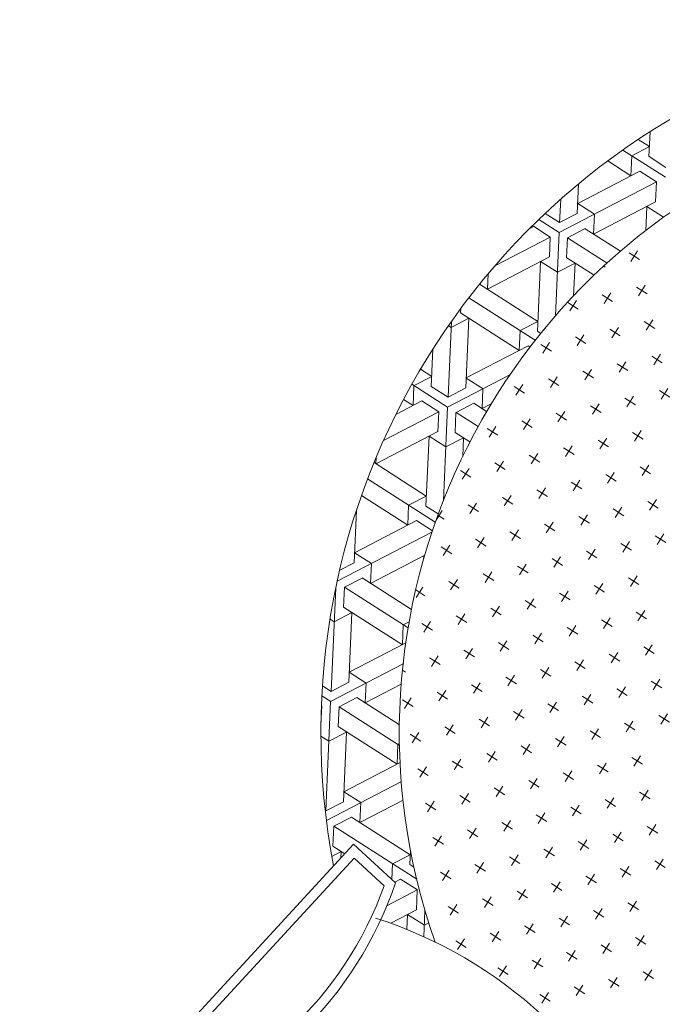
# Model space of a CAD drawing. Units: inches. Extents: x -4843 to -3402, y -164 to 3629.
# Tile 11 of 22: x -4530 to -4506, y 864 to 900. Entities that reach past the tile are written whole.
import ezdxf

# ---------------------------------------------------------------- set-up
doc = ezdxf.new("R2010")
doc.units = ezdxf.units.IN
doc.layers.add('furniture', color=6, linetype='Continuous', lineweight=18)

# ---------------------------------------------------------------- blocks, each defined once
blk = doc.blocks.new('A$C30AE1D3B')
for p, q in [((2071.5, 1090.4, -685.7), (2054.2, 1082.4, -685.7)), ((2066.8, 1077.8, -685.7), (2058.8, 1095.1, -685.7)), ((2122.1, 1072, -685.7), (2104.8, 1064, -685.7)), ((2117.5, 1059.4, -685.7), (2109.4, 1076.6, -685.7)), ((2172.7, 1053.6, -685.7), (2155.5, 1045.5, -685.7)), ((2168.1, 1040.9, -685.7), (2160.1, 1058.2, -685.7)), ((2053, 1039.8, -685.7), (2035.8, 1031.8, -685.7)), ((2048.4, 1027.2, -685.7), (2040.4, 1044.4, -685.7)), ((2218.7, 1022.5, -685.7), (2210.7, 1039.8, -685.7)), ((2099.1, 1008.7, -685.7), (2091, 1026, -685.7)), ((2223.4, 1035.2, -685.7), (2206.1, 1027.1, -685.7)), ((2103.7, 1021.4, -685.7), (2086.4, 1013.3, -685.7)), ((2030, 976.5, -685.7), (2021.9, 993.8, -685.7)), ((2154.3, 1003, -685.7), (2137, 994.9, -685.7)), ((2149.7, 990.3, -685.7), (2141.6, 1007.6, -685.7)), ((2034.6, 989.2, -685.7), (2017.3, 981.1, -685.7)), ((2204.9, 984.5, -685.7), (2187.7, 976.5, -685.7)), ((2200.3, 971.9, -685.7), (2192.3, 989.1, -685.7)), ((2085.2, 970.8, -685.7), (2068, 962.7, -685.7)), ((2080.6, 958.1, -685.7), (2072.6, 975.4, -685.7)), ((2255.6, 966.1, -685.7), (2238.3, 958, -685.7)), ((2250.9, 953.4, -685.7), (2242.9, 970.7, -685.7)), ((1965.5, 957, -685.7), (1948.3, 948.9, -685.7)), ((1960.9, 944.3, -685.7), (1952.9, 961.6, -685.7)), ((2135.9, 952.3, -685.7), (2118.6, 944.3, -685.7)), ((2131.3, 939.7, -685.7), (2123.2, 956.9, -685.7)), ((2016.2, 938.6, -685.7), (1998.9, 930.5, -685.7)), ((2011.6, 925.9, -685.7), (2003.5, 943.2, -685.7)), ((2186.5, 933.9, -685.7), (2169.2, 925.8, -685.7)), ((2181.9, 921.2, -685.7), (2173.8, 938.5, -685.7)), ((2066.8, 920.1, -685.7), (2049.5, 912.1, -685.7)), ((2062.2, 907.5, -685.7), (2054.1, 924.7, -685.7)), ((2232.5, 902.8, -685.7), (2224.5, 920.1, -685.7)), ((1947.1, 906.3, -685.7), (1929.8, 898.3, -685.7)), ((1942.5, 893.7, -685.7), (1934.4, 911, -685.7)), ((2112.8, 889, -685.7), (2104.8, 906.3, -685.7)), ((2237.1, 915.5, -685.7), (2219.9, 907.4, -685.7)), ((1997.7, 887.9, -685.7), (1980.5, 879.9, -685.7)), ((1993.1, 875.3, -685.7), (1985.1, 892.5, -685.7)), ((2117.4, 901.7, -685.7), (2100.2, 893.6, -685.7)), ((2163.5, 870.6, -685.7), (2155.4, 887.9, -685.7)), ((2287.8, 897, -685.7), (2270.5, 889, -685.7)), ((2283.2, 884.4, -685.7), (2275.1, 901.6, -685.7)), ((2043.8, 856.8, -685.7), (2035.7, 874.1, -685.7)), ((2168.1, 883.3, -685.7), (2150.8, 875.2, -685.7)), ((3045.6, 881, -685.7), (2346.6, 694.2, -685.7)), ((1924.1, 843.1, -685.7), (1916, 860.3, -685.7)), ((2048.4, 869.5, -685.7), (2031.1, 861.4, -685.7)), ((2218.7, 864.8, -685.7), (2201.4, 856.8, -685.7)), ((2214.1, 852.2, -685.7), (2206, 869.4, -685.7)), ((3064, 870.4, -685.7), (2336, 675.8, -685.7)), ((1928.7, 855.7, -685.7), (1911.4, 847.7, -685.7)), ((2099, 851.1, -685.7), (2081.7, 843, -685.7)), ((2094.4, 838.4, -685.7), (2086.3, 855.7, -685.7)), ((2269.3, 846.4, -685.7), (2252.1, 838.4, -685.7)), ((2264.7, 833.7, -685.7), (2256.7, 851, -685.7)), ((2298.2, 820.3, -685.7), (2321, 852.9, -685.7)), ((1979.3, 837.3, -685.7), (1962, 829.2, -685.7)), ((1974.7, 824.6, -685.7), (1966.7, 841.9, -685.7)), ((2149.6, 832.6, -685.7), (2132.4, 824.6, -685.7)), ((2145, 820, -685.7), (2137, 837.2, -685.7)), ((2310.8, 838.4, -685.7), (2303.4, 839.1, -685.7)), ((2310.8, 838.4, -685.7), (2323.7, 810.8, -685.7)), ((2336.8, 829.5, -685.7), (2323.7, 810.8, -685.7)), ((2029.9, 818.9, -685.7), (2012.7, 810.8, -685.7)), ((2025.3, 806.2, -685.7), (2017.3, 823.5, -685.7)), ((2200.3, 814.2, -685.7), (2183, 806.2, -685.7)), ((2195.7, 801.5, -685.7), (2187.6, 818.8, -685.7)), ((1910.3, 805.1, -685.7), (1893, 797, -685.7)), ((1905.6, 792.4, -685.7), (1897.6, 809.7, -685.7)), ((2080.6, 800.4, -685.7), (2063.3, 792.4, -685.7)), ((2076, 787.8, -685.7), (2067.9, 805, -685.7)), ((2246.3, 783.1, -685.7), (2238.2, 800.4, -685.7)), ((2291.1, 787.2, -685.7), (2308.5, 812.1, -685.7)), ((2308.5, 812.1, -685.7), (2352.6, 808.3, -685.7)), ((1960.9, 786.7, -685.7), (1943.6, 778.6, -685.7)), ((1956.3, 774, -685.7), (1948.2, 791.3, -685.7)), ((2126.6, 769.3, -685.7), (2118.5, 786.6, -685.7)), ((2250.9, 795.8, -685.7), (2233.6, 787.7, -685.7)), ((2291, 787.2, -685.7), (2303.9, 759.5, -685.7)), ((2343.1, 782.6, -685.7), (2291, 787.1, -685.7)), ((1841.2, 772.9, -685.7), (1823.9, 764.8, -685.7)), ((1836.6, 760.2, -685.7), (1828.5, 777.5, -685.7)), ((2011.5, 768.2, -685.7), (1994.2, 760.2, -685.7)), ((2006.9, 755.6, -685.7), (1998.9, 772.8, -685.7)), ((2131.2, 782, -685.7), (2113.9, 773.9, -685.7)), ((2177.2, 750.9, -685.7), (2169.2, 768.2, -685.7)), ((2283.1, 772.9, -685.7), (2346.7, 636.6, -685.7)), ((1891.8, 754.5, -685.7), (1874.6, 746.4, -685.7)), ((1887.2, 741.8, -685.7), (1879.2, 759.1, -685.7)), ((2057.5, 737.1, -685.7), (2049.5, 754.4, -685.7)), ((2181.8, 763.6, -685.7), (2164.6, 755.5, -685.7)), ((2276.8, 755.2, -685.7), (2280, 748.4, -685.7)), ((2301.6, 733.2, -685.7), (2315.4, 752.9, -685.7)), ((2303.9, 759.5, -685.7), (2313.8, 758.7, -685.7)), ((2336, 675.8, -685.7), (2313.4, 760.3, -685.7)), ((2346.6, 694.2, -685.7), (2330.4, 754.6, -685.7)), ((1937.8, 723.4, -685.7), (1929.8, 740.6, -685.7)), ((2062.1, 749.8, -685.7), (2044.9, 741.7, -685.7)), ((2232.5, 745.1, -685.7), (2215.2, 737.1, -685.7)), ((2227.9, 732.5, -685.7), (2219.8, 749.8, -685.7)), ((2280, 748.4, -685.7), (2267.2, 730.1, -685.7)), ((1822.8, 722.2, -685.7), (1805.5, 714.2, -685.7)), ((1818.2, 709.6, -685.7), (1810.1, 726.9, -685.7)), ((1942.5, 736, -685.7), (1925.2, 728, -685.7)), ((2112.8, 731.4, -685.7), (2095.5, 723.3, -685.7)), ((2108.2, 718.7, -685.7), (2100.1, 736, -685.7)), ((2316.3, 639.2, -685.7), (2271.3, 735.9, -685.7)), ((2301.6, 733.2, -685.7), (2271.3, 735.9, -685.7)), ((1868.8, 691.2, -685.7), (1860.7, 708.4, -685.7)), ((1993.1, 717.6, -685.7), (1975.8, 709.5, -685.7)), ((1988.5, 704.9, -685.7), (1980.4, 722.2, -685.7)), ((2163.4, 712.9, -685.7), (2146.1, 704.9, -685.7)), ((2158.8, 700.3, -685.7), (2150.8, 717.5, -685.7)), ((1873.4, 703.8, -685.7), (1856.1, 695.8, -685.7)), ((2043.7, 699.2, -685.7), (2026.5, 691.1, -685.7)), ((2039.1, 686.5, -685.7), (2031.1, 703.8, -685.7)), ((2214, 694.5, -685.7), (2196.8, 686.5, -685.7)), ((2209.4, 681.9, -685.7), (2201.4, 699.1, -685.7)), ((1924, 685.4, -685.7), (1906.8, 677.3, -685.7)), ((1919.4, 672.7, -685.7), (1911.4, 690, -685.7)), ((2094.4, 680.7, -685.7), (2077.1, 672.7, -685.7)), ((2089.7, 668.1, -685.7), (2081.7, 685.3, -685.7)), ((2364.2, 661.5, -685.7), (2355.1, 681, -685.7)), ((2363.2, 683.1, -685.7), (2357.8, 675.3, -685.7)), ((1804.3, 671.6, -685.7), (1787.1, 663.6, -685.7)), ((1799.7, 659, -685.7), (1791.7, 676.2, -685.7)), ((1974.7, 667, -685.7), (1957.4, 658.9, -685.7)), ((1970.1, 654.3, -685.7), (1962, 671.6, -685.7)), ((2145, 662.3, -685.7), (2127.7, 654.3, -685.7)), ((2140.4, 649.6, -685.7), (2132.3, 666.9, -685.7)), ((2373.9, 673.9, -685.7), (2357.8, 675.3, -685.7)), ((1855, 653.2, -685.7), (1837.7, 645.1, -685.7)), ((1850.4, 640.5, -685.7), (1842.3, 657.8, -685.7)), ((2025.3, 648.5, -685.7), (2008, 640.5, -685.7)), ((2020.7, 635.9, -685.7), (2012.6, 653.1, -685.7)), ((2191, 631.2, -685.7), (2183, 648.5, -685.7)), ((2235.7, 659.5, -685.7), (2309.9, 653, -685.7)), ((2292.4, 628.1, -685.7), (2309.9, 653, -685.7)), ((2346.7, 636.6, -685.7), (2364.2, 661.5, -685.7)), ((1905.6, 634.8, -685.7), (1888.3, 626.7, -685.7)), ((1901, 622.1, -685.7), (1892.9, 639.4, -685.7)), ((2071.3, 617.4, -685.7), (2063.3, 634.7, -685.7)), ((2195.6, 643.9, -685.7), (2178.3, 635.8, -685.7)), ((2351.3, 622.9, -685.7), (2222.7, 634.1, -685.7)), ((2346.7, 636.5, -685.7), (2316.3, 639.2, -685.7)), ((1785.9, 621, -685.7), (1768.6, 612.9, -685.7)), ((1781.3, 608.3, -685.7), (1773.2, 625.6, -685.7)), ((1951.6, 603.7, -685.7), (1943.6, 620.9, -685.7)), ((2075.9, 630.1, -685.7), (2058.7, 622.1, -685.7)), ((2292.4, 628.1, -685.7), (2305.3, 600.4, -685.7)), ((1836.5, 602.6, -685.7), (1819.3, 594.5, -685.7)), ((1831.9, 589.9, -685.7), (1823.9, 607.2, -685.7)), ((1956.2, 616.3, -685.7), (1939, 608.3, -685.7)), ((2002.3, 585.2, -685.7), (1994.2, 602.5, -685.7)), ((2126.6, 611.7, -685.7), (2109.3, 603.6, -685.7)), ((2121.9, 599, -685.7), (2113.9, 616.3, -685.7)), ((2196.7, 583.4, -685.7), (2214.2, 608.4, -685.7)), ((2208.8, 608.9, -685.7), (2305.3, 600.4, -685.7)), ((2259.3, 511.7, -685.7), (2214.2, 608.4, -685.7)), ((2248.3, 472.9, -685.7), (2344.4, 610.3, -685.7)), ((2314.1, 612.9, -685.7), (2252.9, 525.5, -685.7)), ((2344.4, 610.2, -685.7), (2314, 612.9, -685.7)), ((2344.4, 610.3, -685.7), (2344.8, 609.4, -685.7)), ((1882.6, 571.5, -685.7), (1874.5, 588.7, -685.7)), ((2006.9, 597.9, -685.7), (1989.6, 589.8, -685.7)), ((2177.2, 593.2, -685.7), (2159.9, 585.2, -685.7)), ((2172.6, 580.6, -685.7), (2164.5, 597.9, -685.7)), ((1762.9, 557.7, -685.7), (1754.8, 575, -685.7)), ((1887.2, 584.1, -685.7), (1869.9, 576.1, -685.7)), ((2057.5, 579.5, -685.7), (2040.2, 571.4, -685.7)), ((2052.9, 566.8, -685.7), (2044.8, 584.1, -685.7)), ((2196.7, 583.4, -685.7), (2193.9, 583.7, -685.7)), ((2195.4, 586.2, -685.7), (2241.8, 486.8, -685.7)), ((1767.5, 570.4, -685.7), (1750.2, 562.3, -685.7)), ((1937.8, 565.7, -685.7), (1920.5, 557.6, -685.7)), ((1933.2, 553, -685.7), (1925.1, 570.3, -685.7)), ((2108.1, 561, -685.7), (2090.9, 553, -685.7)), ((2103.5, 548.4, -685.7), (2095.5, 565.7, -685.7)), ((2211.4, 489.4, -685.7), (2178.7, 559.6, -685.7)), ((1693.8, 525.5, -685.7), (1685.8, 542.8, -685.7)), ((1818.1, 551.9, -685.7), (1800.8, 543.9, -685.7)), ((1813.5, 539.3, -685.7), (1805.4, 556.5, -685.7)), ((1988.4, 547.3, -685.7), (1971.2, 539.2, -685.7)), ((1983.8, 534.6, -685.7), (1975.8, 551.9, -685.7)), ((2158.8, 542.6, -685.7), (2141.5, 534.6, -685.7)), ((2154.2, 530, -685.7), (2146.1, 547.2, -685.7)), ((1698.4, 538.1, -685.7), (1681.2, 530.1, -685.7)), ((1868.7, 533.5, -685.7), (1851.5, 525.4, -685.7)), ((1864.1, 520.8, -685.7), (1856.1, 538.1, -685.7)), ((2039.1, 528.8, -685.7), (2021.8, 520.8, -685.7)), ((2034.5, 516.2, -685.7), (2026.4, 533.4, -685.7)), ((1749, 519.7, -685.7), (1731.8, 511.7, -685.7)), ((1744.4, 507.1, -685.7), (1736.4, 524.3, -685.7)), ((1919.4, 515.1, -685.7), (1902.1, 507, -685.7)), ((1914.8, 502.4, -685.7), (1906.7, 519.7, -685.7)), ((2085.1, 497.8, -685.7), (2077, 515, -685.7)), ((2241.8, 486.7, -685.7), (2259.3, 511.7, -685.7)), ((2283.2, 522.9, -685.7), (2252.9, 525.5, -685.7)), ((2283.2, 522.9, -685.7), (2289.3, 509.8, -685.7)), ((1799.7, 501.3, -685.7), (1782.4, 493.2, -685.7)), ((1795.1, 488.6, -685.7), (1787, 505.9, -685.7)), ((1970, 496.6, -685.7), (1952.7, 488.6, -685.7)), ((1965.4, 484, -685.7), (1957.3, 501.2, -685.7)), ((2089.7, 510.4, -685.7), (2072.4, 502.4, -685.7)), ((2130, 491.6, -685.7), (2127.7, 496.6, -685.7)), ((2143, 508.6, -685.7), (2205, 503.2, -685.7)), ((2187.5, 478.2, -685.7), (2205, 503.2, -685.7)), ((1680, 487.5, -685.7), (1662.7, 479.5, -685.7)), ((1675.4, 474.9, -685.7), (1667.3, 492.1, -685.7)), ((1850.3, 482.9, -685.7), (1833, 474.8, -685.7)), ((1845.7, 470.2, -685.7), (1837.7, 487.5, -685.7)), ((2016, 465.5, -685.7), (2008, 482.8, -685.7)), ((2124.4, 484.6, -685.7), (2123.1, 483.9, -685.7)), ((2248.3, 472.9, -685.7), (2123.8, 483.8, -685.7)), ((2241.8, 486.7, -685.7), (2211.4, 489.4, -685.7)), ((2263.5, 471.6, -685.7), (2279.6, 494.6, -685.7)), ((1730.6, 469.1, -685.7), (1713.4, 461, -685.7)), ((1726, 456.4, -685.7), (1718, 473.7, -685.7)), ((1896.3, 451.8, -685.7), (1888.3, 469, -685.7)), ((2020.6, 478.2, -685.7), (2003.4, 470.2, -685.7)), ((2187.5, 478.3, -685.7), (2200.4, 450.6, -685.7)), ((2248.2, 472.9, -685.7), (2255, 458.5, -685.7)), ((2263.4, 471.6, -685.7), (2263.7, 471, -685.7)), ((2264.1, 471.5, -685.7), (2263.4, 471.6, -685.7)), ((1776.6, 438, -685.7), (1768.6, 455.3, -685.7)), ((1900.9, 464.4, -685.7), (1883.7, 456.4, -685.7)), ((2071.3, 459.8, -685.7), (2054, 451.7, -685.7)), ((2066.7, 447.1, -685.7), (2058.6, 464.4, -685.7)), ((2091.8, 433.6, -685.7), (2109.3, 458.6, -685.7)), ((2103.4, 459.1, -685.7), (2200.4, 450.6, -685.7)), ((2154.4, 361.9, -685.7), (2109.3, 458.6, -685.7)), ((2209.2, 463.1, -685.7), (2148, 375.7, -685.7)), ((2148.8, 330.8, -685.7), (2239.5, 460.5, -685.7)), ((2239.5, 460.4, -685.7), (2209.1, 463.1, -685.7)), ((2239.5, 460.5, -685.7), (2246.1, 446.2, -685.7)), ((1661.6, 436.9, -685.7), (1644.3, 428.8, -685.7)), ((1657, 424.2, -685.7), (1648.9, 441.5, -685.7)), ((1781.3, 450.7, -685.7), (1764, 442.6, -685.7)), ((1827.3, 419.6, -685.7), (1819.2, 436.8, -685.7)), ((1951.6, 446, -685.7), (1934.3, 438, -685.7)), ((1947, 433.3, -685.7), (1938.9, 450.6, -685.7)), ((2088.1, 441.7, -685.7), (2136.9, 336.9, -685.7)), ((1707.6, 405.8, -685.7), (1699.5, 423.1, -685.7)), ((1831.9, 432.2, -685.7), (1814.6, 424.2, -685.7)), ((2002.2, 427.6, -685.7), (1984.9, 419.5, -685.7)), ((1997.6, 414.9, -685.7), (1989.5, 432.2, -685.7)), ((2091.8, 433.6, -685.7), (2081.6, 434.5, -685.7)), ((1712.2, 418.5, -685.7), (1694.9, 410.4, -685.7)), ((1882.5, 413.8, -685.7), (1865.2, 405.7, -685.7)), ((1877.9, 401.1, -685.7), (1869.9, 418.4, -685.7)), ((2052.8, 409.1, -685.7), (2035.6, 401.1, -685.7)), ((2047.2, 398.8, -685.7), (2040.2, 413.8, -685.7)), ((2106.5, 339.6, -685.7), (2068.7, 420.7, -685.7)), ((1762.8, 400, -685.7), (1745.6, 392, -685.7)), ((1758.2, 387.4, -685.7), (1750.2, 404.6, -685.7)), ((1933.1, 395.4, -685.7), (1915.9, 387.3, -685.7)), ((1928.5, 382.7, -685.7), (1920.5, 400, -685.7)), ((1643.1, 386.3, -685.7), (1625.9, 378.2, -685.7)), ((1638.5, 373.6, -685.7), (1630.5, 390.9, -685.7)), ((1813.5, 381.6, -685.7), (1796.2, 373.5, -685.7)), ((1808.8, 368.9, -685.7), (1800.8, 386.2, -685.7)), ((1983.8, 376.9, -685.7), (1966.5, 368.9, -685.7)), ((1979.2, 364.3, -685.7), (1971.1, 381.6, -685.7)), ((1693.8, 367.8, -685.7), (1676.5, 359.8, -685.7)), ((1689.2, 355.2, -685.7), (1681.1, 372.4, -685.7)), ((1864.1, 363.2, -685.7), (1846.8, 355.1, -685.7)), ((1859.5, 350.5, -685.7), (1851.4, 367.8, -685.7)), ((2007.1, 361.5, -685.7), (2100.1, 353.4, -685.7)), ((2008.4, 362.7, -685.7), (2009, 361.4, -685.7)), ((2012.4, 366.2, -685.7), (2009, 361.4, -685.7)), ((2136.9, 336.9, -685.7), (2154.4, 361.9, -685.7)), ((2178.3, 373.1, -685.7), (2148, 375.7, -685.7)), ((2178.3, 373.1, -685.7), (2181.5, 366.2, -685.7)), ((1574.1, 354, -685.7), (1556.8, 346, -685.7)), ((1569.5, 341.4, -685.7), (1561.4, 358.7, -685.7)), ((1744.4, 349.4, -685.7), (1727.1, 341.3, -685.7)), ((1739.8, 336.7, -685.7), (1731.7, 354, -685.7)), ((1910.1, 332.1, -685.7), (1902.1, 349.3, -685.7)), ((2082.6, 328.4, -685.7), (2100.1, 353.4, -685.7)), ((1624.7, 335.6, -685.7), (1607.4, 327.6, -685.7)), ((1620.1, 323, -685.7), (1612, 340.2, -685.7)), ((1790.4, 318.3, -685.7), (1782.4, 335.6, -685.7)), ((1914.7, 344.7, -685.7), (1897.5, 336.7, -685.7)), ((1977.1, 336.2, -685.7), (1989.2, 310.1, -685.7)), ((2141.4, 323.3, -685.7), (1978.8, 337.5, -685.7)), ((2136.9, 336.9, -685.7), (2106.6, 339.6, -685.7)), ((1675.3, 317.2, -685.7), (1658.1, 309.1, -685.7)), ((1670.7, 304.5, -685.7), (1662.7, 321.8, -685.7)), ((1795, 331, -685.7), (1777.8, 322.9, -685.7)), ((1841.1, 299.9, -685.7), (1833, 317.1, -685.7)), ((1963.8, 325.6, -685.7), (1948.1, 318.3, -685.7)), ((1957.5, 320.7, -685.7), (1952.7, 330.9, -685.7)), ((1955.8, 319.4, -685.7), (1965.3, 299, -685.7)), ((1966.5, 327.7, -685.7), (2018.4, 216.3, -685.7)), ((2082.6, 328.4, -685.7), (2095.5, 300.8, -685.7)), ((1555.6, 303.4, -685.7), (1538.4, 295.4, -685.7)), ((1551, 290.8, -685.7), (1543, 308, -685.7)), ((1721.4, 286.1, -685.7), (1713.3, 303.4, -685.7)), ((1845.7, 312.5, -685.7), (1828.4, 304.5, -685.7)), ((1856.3, 189.3, -685.7), (1938.2, 306.3, -685.7)), ((1987, 283.8, -685.7), (2004.4, 308.8, -685.7)), ((1989.2, 310.1, -685.7), (2095.5, 300.8, -685.7)), ((2039.9, 232.7, -685.7), (2004.4, 308.8, -685.7)), ((2104.3, 313.3, -685.7), (2058.1, 247.4, -685.7)), ((2129.1, 311.1, -685.7), (2104.3, 313.3, -685.7)), ((1601.7, 272.3, -685.7), (1593.6, 289.6, -685.7)), ((1726, 298.8, -685.7), (1708.7, 290.7, -685.7)), ((1896.3, 294.1, -685.7), (1879, 286.1, -685.7)), ((1891.7, 281.5, -685.7), (1883.6, 298.7, -685.7)), ((1965.3, 299, -685.7), (1904.1, 211.6, -685.7)), ((1996.7, 200.5, -685.7), (1956.6, 286.5, -685.7)), ((1986.9, 283.8, -685.7), (1956.6, 286.5, -685.7)), ((1606.3, 285, -685.7), (1589, 276.9, -685.7)), ((1652.3, 253.9, -685.7), (1644.2, 271.2, -685.7)), ((1776.6, 280.3, -685.7), (1759.3, 272.3, -685.7)), ((1772, 267.7, -685.7), (1763.9, 284.9, -685.7)), ((1532.6, 240.1, -685.7), (1524.6, 257.4, -685.7)), ((1656.9, 266.6, -685.7), (1639.6, 258.5, -685.7)), ((1827.2, 261.9, -685.7), (1810, 253.9, -685.7)), ((1822.6, 249.2, -685.7), (1814.6, 266.5, -685.7)), ((1877.3, 265.3, -685.7), (1860.9, 241.9, -685.7)), ((1537.2, 252.8, -685.7), (1519.9, 244.7, -685.7)), ((1707.5, 248.1, -685.7), (1690.3, 240.1, -685.7)), ((1702.9, 235.5, -685.7), (1694.9, 252.7, -685.7)), ((1867.3, 228, -685.7), (1856, 252.4, -685.7)), ((1891.2, 239.2, -685.7), (1860.9, 241.8, -685.7)), ((1587.8, 234.4, -685.7), (1570.6, 226.3, -685.7)), ((1583.2, 221.7, -685.7), (1575.2, 239, -685.7)), ((1758.2, 229.7, -685.7), (1740.9, 221.7, -685.7)), ((1753.6, 217, -685.7), (1745.5, 234.3, -685.7)), ((1819.5, 205.7, -685.7), (1809.6, 227, -685.7)), ((1832.9, 239.4, -685.7), (1849.8, 203.1, -685.7)), ((1849.9, 203.1, -685.7), (1867.3, 228, -685.7)), ((1891.2, 239.2, -685.7), (1904.1, 211.6, -685.7)), ((1638.5, 215.9, -685.7), (1621.2, 207.9, -685.7)), ((1633.9, 203.3, -685.7), (1625.8, 220.5, -685.7)), ((1795.6, 194.6, -685.7), (1813.1, 219.5, -685.7)), ((1797.5, 220.9, -685.7), (1813, 219.5, -685.7)), ((1871.5, 187.9, -685.7), (1889, 212.9, -685.7)), ((1888.9, 212.9, -685.7), (1995.2, 203.6, -685.7)), ((1518.8, 202.2, -685.7), (1501.5, 194.1, -685.7)), ((1514.2, 189.5, -685.7), (1506.1, 206.8, -685.7)), ((1689.1, 197.5, -685.7), (1671.8, 189.4, -685.7)), ((1684.5, 184.8, -685.7), (1676.4, 202.1, -685.7)), ((1856.3, 189.2, -685.7), (1749.3, 198.6, -685.7)), ((1849.8, 203.1, -685.7), (1819.5, 205.7, -685.7)), ((1989.6, 195.5, -685.7), (1995.2, 203.6, -685.7)), ((1569.4, 183.7, -685.7), (1552.2, 175.7, -685.7)), ((1564.8, 171.1, -685.7), (1556.8, 188.3, -685.7)), ((1795.5, 194.6, -685.7), (1808.4, 167, -685.7)), ((1856.3, 189.3, -685.7), (1883.7, 130.4, -685.7)), ((1871.5, 187.9, -685.7), (1884.3, 160.3, -685.7)), ((1966.1, 179.6, -685.7), (1871.5, 187.9, -685.7)), ((1615.4, 152.6, -685.7), (1607.4, 169.9, -685.7)), ((1675.7, 170.5, -685.7), (1678.2, 165.1, -685.7)), ((1688.3, 174.8, -685.7), (1739.2, 65.6, -685.7)), ((1699.9, 150, -685.7), (1717.4, 174.9, -685.7)), ((1700.7, 179.3, -685.7), (1702.2, 176.3, -685.7)), ((1702.2, 176.2, -685.7), (1808.4, 166.9, -685.7)), ((1762.4, 78.2, -685.7), (1717.3, 174.9, -685.7)), ((1817.2, 179.4, -685.7), (1756, 92, -685.7)), ((1781.1, 81.8, -685.7), (1847.6, 176.8, -685.7)), ((1847.5, 176.8, -685.7), (1817.2, 179.4, -685.7)), ((1847.5, 176.8, -685.7), (1860.4, 149.2, -685.7)), ((1500.4, 151.5, -685.7), (1483.1, 143.5, -685.7)), ((1495.7, 138.9, -685.7), (1487.7, 156.1, -685.7)), ((1569.2, 55.4, -685.7), (1642.5, 160, -685.7)), ((1620, 165.3, -685.7), (1602.8, 157.2, -685.7)), ((1678.3, 165.1, -685.7), (1617.1, 77.7, -685.7)), ((1699.9, 149.9, -685.7), (1669.5, 152.6, -685.7)), ((1714.2, 56.8, -685.7), (1669.5, 152.6, -685.7)), ((1882.1, 134, -685.7), (1899.5, 159, -685.7)), ((1884.3, 160.3, -685.7), (1929.2, 156.4, -685.7)), ((1906.9, 143.2, -685.7), (1899.5, 159, -685.7)), ((1539.4, 135.5, -685.7), (1538.3, 137.7, -685.7)), ((1580.2, 94.2, -685.7), (1559.2, 139.3, -685.7)), ((1602.6, 149.1, -685.7), (1573.8, 108, -685.7)), ((1860.4, 149.2, -685.7), (1827.6, 102.2, -685.7)), ((1860.3, 118.2, -685.7), (1851.7, 136.7, -685.7)), ((1882, 134, -685.7), (1851.7, 136.7, -685.7)), ((1422, 121.3, -685.7), (1434.9, 93.7, -685.7)), ((1456.2, 124.1, -685.7), (1434.9, 93.6, -685.7)), ((1532.4, 71.9, -685.7), (1505.3, 129.9, -685.7)), ((1532.4, 134.2, -685.7), (1562.8, 69.2, -685.7)), ((1604.2, 105.3, -685.7), (1573.8, 108, -685.7)), ((1604.2, 105.3, -685.7), (1617, 77.7, -685.7)), ((1402.2, 70, -685.7), (1419.7, 95, -685.7)), ((1419.7, 95, -685.7), (1526, 85.7, -685.7)), ((1562.8, 69.2, -685.7), (1580.3, 94.2, -685.7)), ((1786.3, 89.4, -685.7), (1756, 92, -685.7)), ((1508.5, 60.7, -685.7), (1526, 85.7, -685.7)), ((1584.4, 54.1, -685.7), (1601.9, 79, -685.7)), ((1601.9, 79, -685.7), (1708.1, 69.7, -685.7)), ((1758.7, 72.9, -685.7), (1762.4, 78.2, -685.7)), ((1786.3, 89.4, -685.7), (1788.5, 84.9, -685.7)), ((1387, 71.3, -685.7), (1419.7, 1.3, -685.7)), ((1402.2, 70, -685.7), (1415.1, 42.4, -685.7)), ((1569.2, 55.4, -685.7), (1402.2, 70, -685.7)), ((1508.5, 60.7, -685.7), (1521.3, 33.1, -685.7)), ((1562.8, 69.2, -685.7), (1532.4, 71.8, -685.7)), ((1694.7, 50.5, -685.7), (1708.2, 69.7, -685.7)), ((1378.3, 58.9, -685.7), (1391.1, 31.2, -685.7)), ((1530.1, 45.6, -685.7), (1504.3, 8.7, -685.7)), ((1560.5, 42.9, -685.7), (1530.1, 45.6, -685.7)), ((1569.2, 55.4, -685.7), (1584.8, 22, -685.7)), ((1584.4, 54.1, -685.7), (1597.3, 26.4, -685.7)), ((1679.3, 45.7, -685.7), (1584.4, 54.1, -685.7)), ((1391.2, 31.2, -685.7), (1369.3, 0, -685.7)), ((1412.8, 16.1, -685.7), (1430.3, 41.1, -685.7)), ((1415.1, 42.4, -685.7), (1521.4, 33.1, -685.7)), ((1448, 3, -685.7), (1430.3, 41.1, -685.7)), ((1540.1, 13.9, -685.7), (1560.5, 42.9, -685.7)), ((1560.5, 42.9, -685.7), (1571.4, 19.4, -685.7)), ((1391, 0.3, -685.7), (1382.4, 18.7, -685.7)), ((1412.8, 16.1, -685.7), (1382.4, 18.7, -685.7)), ((1597.3, 26.4, -685.7), (1603.1, 25.9, -685.7))]:
    blk.add_line(p, q)
for centre, radius, start, end in [((2899.7, 1230.2, -685.7), 690.9, 170.2555, 219.6682), ((1366.9, 1089.4, -685.7), 1089.4, 168.469, 338.3492), ((1366.9, 1089.4, -685.7), 969.4, 168.0362, 346.8505), ((2677.3, 306.6, -685.7), 581.6, 75.1733, 128.7306), ((2677.3, 306.6, -685.7), 566.6, 73.8832, 127.7449)]:
    blk.add_arc(centre, radius, start, end)

msp = doc.modelspace()

# ---------------------------------------------------------------- block references
at = {"layer": 'furniture', "xscale": 0.0242257431082848, "yscale": 0.0242257431082848, "zscale": 0.0242257431082848, "rotation": 212.4298414976532}
msp.add_blockref('A$C30AE1D3B', (-4478.842, 914.005, -463.669), dxfattribs=at)

doc.saveas('drawing.dxf')
